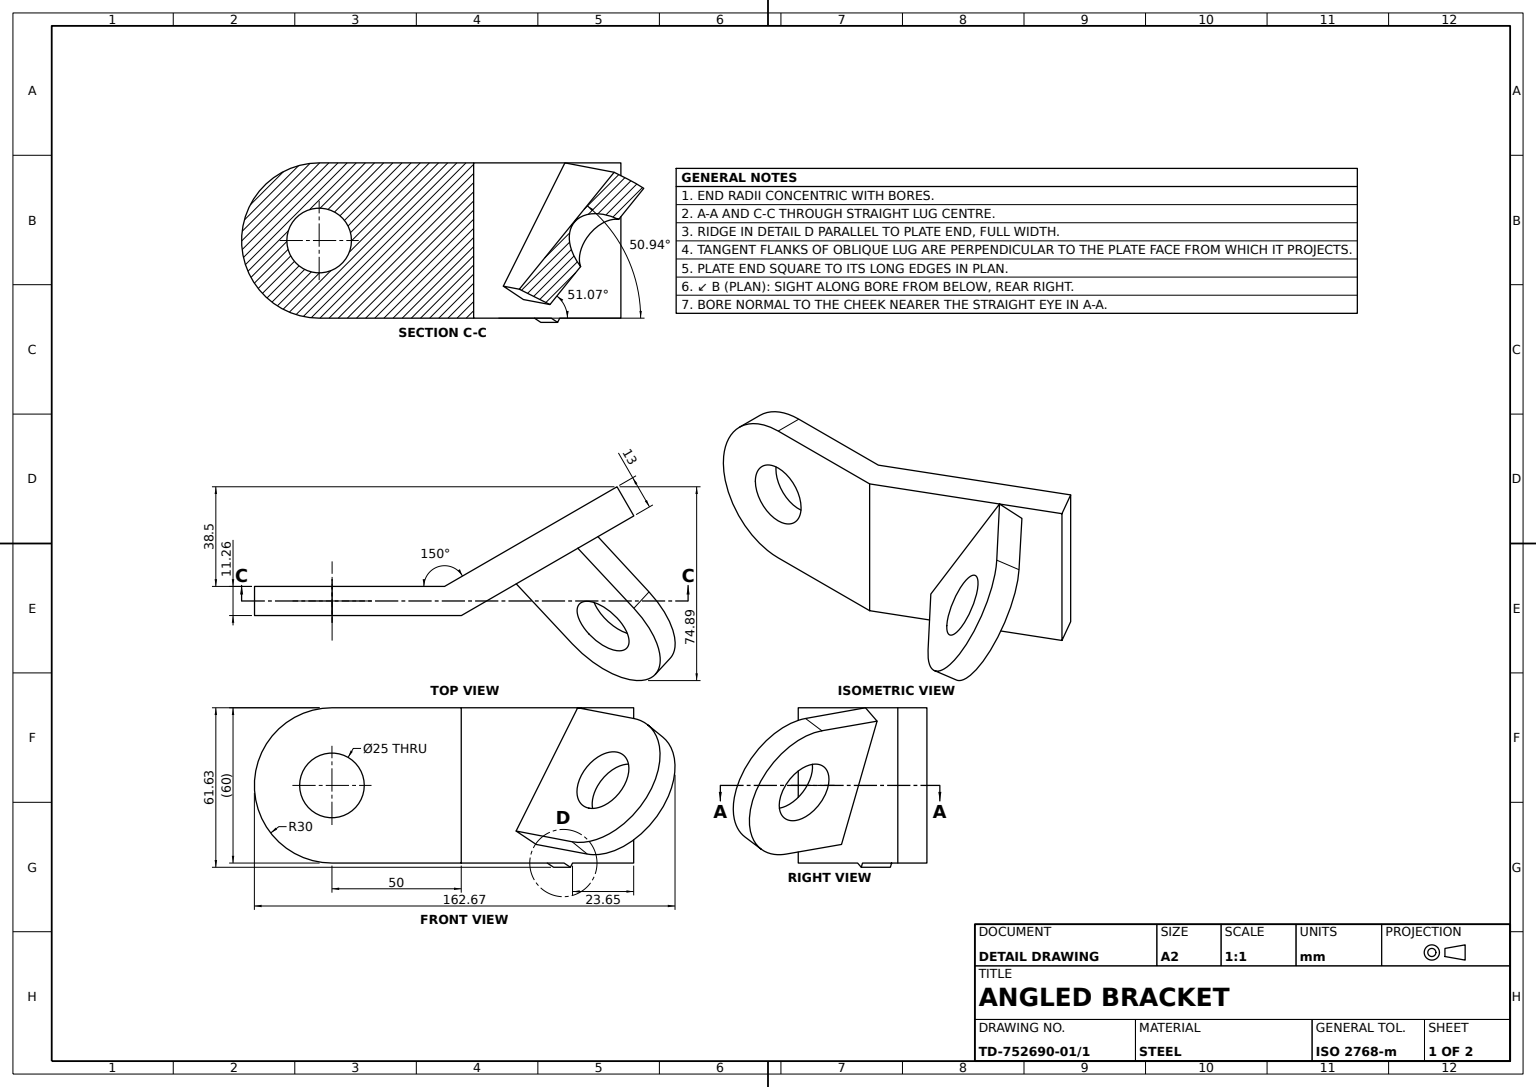
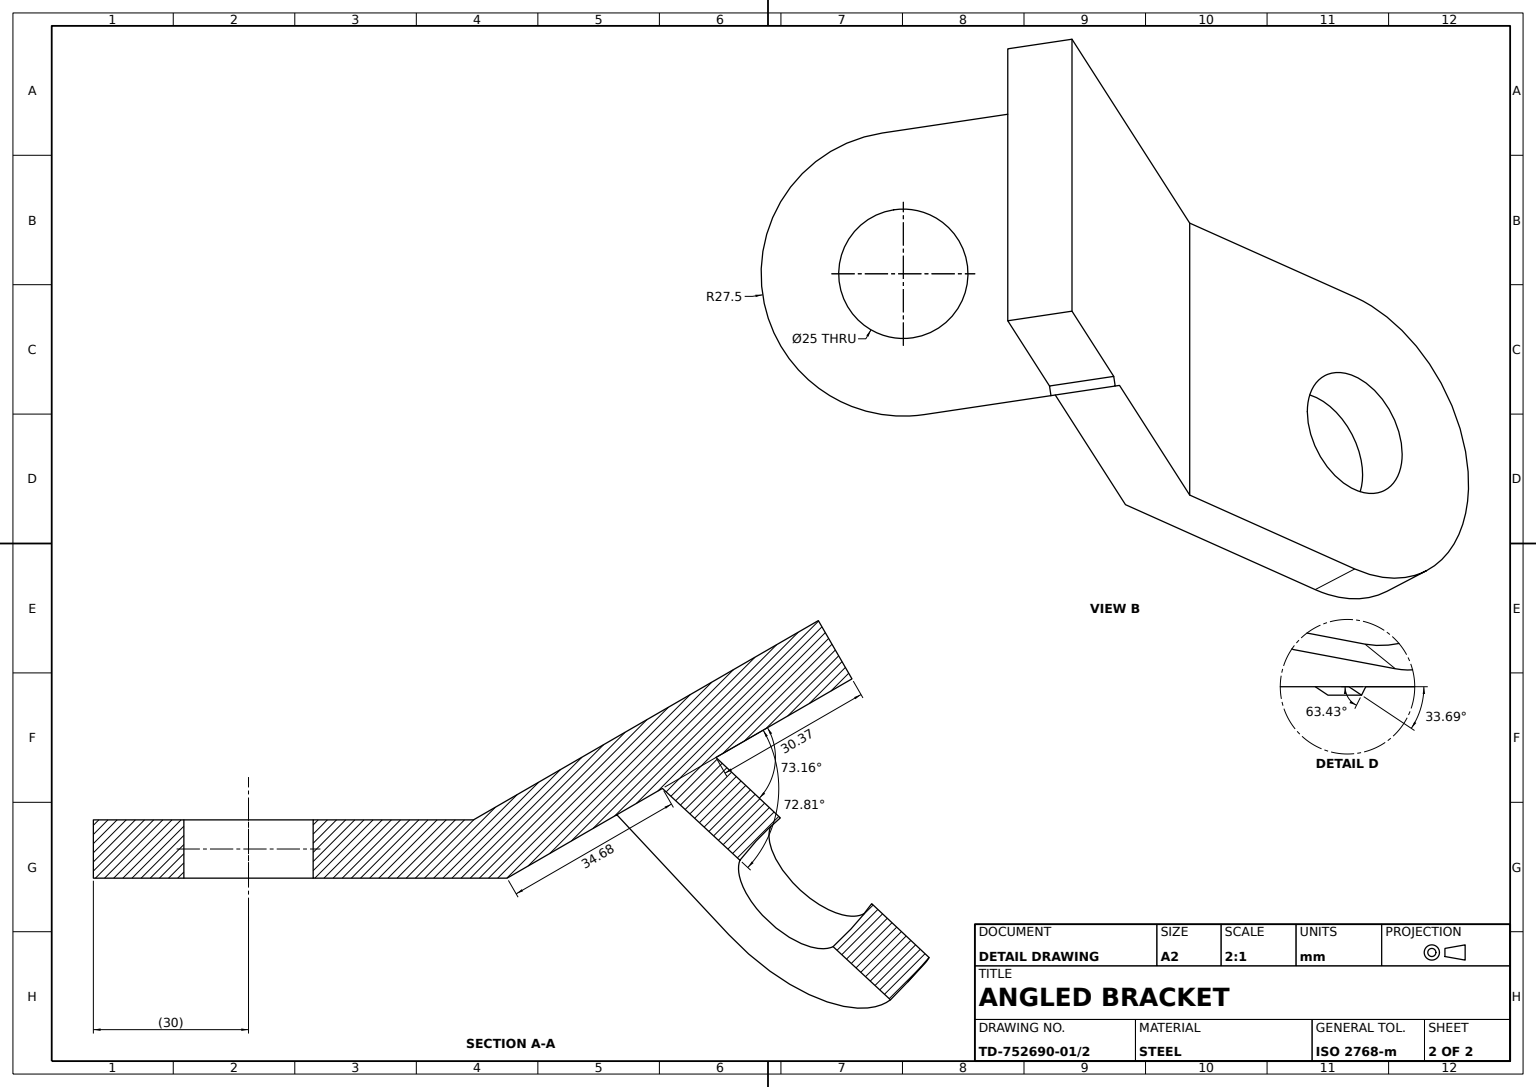
from build123d import *

# Parameters (mm, degrees)
BASE_PLATE_SKETCH_W         = 77
BASE_PLATE_SKETCH_H         = 60
BASE_PLATE_60X77X13_DEPTH   = 13
UPPER_EYE_LUG_DEPTH         = 30
UPPER_LUG_CUT_SKETCH_R      = 12.5
UPPER_LUG_CUT_DEPTH         = 13
LOWER_EYE_LUG_DEPTH         = 13
LOWER_EYE_LUG_DEPTH_BACK    = 62
LOWER_LUG_PROFILE_CUT_DEPTH = 62
LOWER_LUG_TRIM_SKETCH_R     = 12.5
LOWER_LUG_TRIM_CUT_DEPTH    = 62


with BuildPart() as part:
    # Base Plate Sketch → Base Plate 60x77x13 (new body)
    with BuildSketch(Plane.XY):
        Rectangle(BASE_PLATE_SKETCH_W, BASE_PLATE_SKETCH_H)
    extrude(amount=BASE_PLATE_60X77X13_DEPTH)

    # Upper Lug Sketch → Upper Eye Lug (add, symmetric)
    with BuildSketch(Plane(origin=(0, 0, 0), x_dir=(1, 0, 0), z_dir=(0, 1, 0))):
        Polygon((38.5, -13), (38.5, 0), (120.77241336, -47.5), (112.112159322, -55.5), align=None)
    extrude(amount=UPPER_EYE_LUG_DEPTH, both=True)

    # Upper Lug Cut Sketch → Upper Lug Cut (cut)
    with BuildSketch(Plane(origin=(9.625, 0, -16.670989023), x_dir=(-0.8660254037844419, 0, -0.49999999999999434), z_dir=(0.49999999999999434, 0, -0.8660254037844419))):
        with BuildLine():
            Line((-128.341978046, 30), (-128.341978046, -30))
            Line((-128.341978046, -30), (-83.341978046, -30))
            ThreePointArc((-83.341978046, -30), (-113.341978046, 0), (-83.341978046, 30))
            Line((-83.341978046, 30), (-128.341978046, 30))
        make_face()
        with Locations((-83.341978046, 0)):
            Circle(UPPER_LUG_CUT_SKETCH_R)
    extrude(amount=-UPPER_LUG_CUT_DEPTH, mode=Mode.SUBTRACT)

    # Lower Lug Sketch → Lower Eye Lug (add, two sides: drawn at the far end of the back side and taken through both)
    with BuildSketch(Plane.XY.offset(-LOWER_EYE_LUG_DEPTH_BACK)):
        Polygon((14, -17.631397208), (-10.248711306, -31.631397208), (-37.748711306, 16), (-13.5, 30), align=None)
    extrude(amount=LOWER_EYE_LUG_DEPTH + LOWER_EYE_LUG_DEPTH_BACK)

    # Lower Lug Profile Cut Sketch → Lower Lug Profile Cut (cut)
    with BuildSketch(Plane(origin=(-16.365381057, 28.345671476, 0), x_dir=(0.8660254037844398, 0.4999999999999981, 0), z_dir=(-0.49999999999999817, 0.8660254037844398, 0))):
        Polygon((-7.044104755, 0), (-22.768294497, 60), (-12.768294497, 60), (3.308657049, 0), (3.308657049, 62), (-24.691342951, 62), (-24.691342951, 0), align=None)
    extrude(amount=-LOWER_LUG_PROFILE_CUT_DEPTH, mode=Mode.SUBTRACT)

    # Lower Lug Trim Sketch → Lower Lug Trim Cut (cut)
    with BuildSketch(Plane(origin=(2.673436922, 1.543509526, -0.827164262), x_dir=(-0.22414386804201733, -0.129409522551262, -0.9659258262890672), z_dir=(0.836516303737808, 0.48296291314453194, -0.258819045102525))):
        with BuildLine():
            Line((31.143656542, -22.269237886), (61.260227367, -22.269237886))
            Line((61.260227367, -22.269237886), (61.260227367, 32.730762114))
            Line((61.260227367, 32.730762114), (31.143656542, 32.730762114))
            ThreePointArc((31.143656542, 32.730762114), (50.589093025, 24.676198596), (58.643656542, 5.230762114))
            ThreePointArc((58.643656542, 5.230762114), (50.589093025, -14.214674369), (31.143656542, -22.269237886))
        make_face()
        with Locations(Location((31.143656542, 5.230762114, 0), (0, 0, 90))):
            Circle(LOWER_LUG_TRIM_SKETCH_R)
    extrude(amount=-LOWER_LUG_TRIM_CUT_DEPTH, mode=Mode.SUBTRACT)


with BuildPart() as body_2:
    # of the pieces the cut leaves, the one that is kept (lower_lug_trim_cut_keep)
    add(part.part.solids().sort_by_distance((-38.5, 30, 0))[0])


solid = body_2.part
